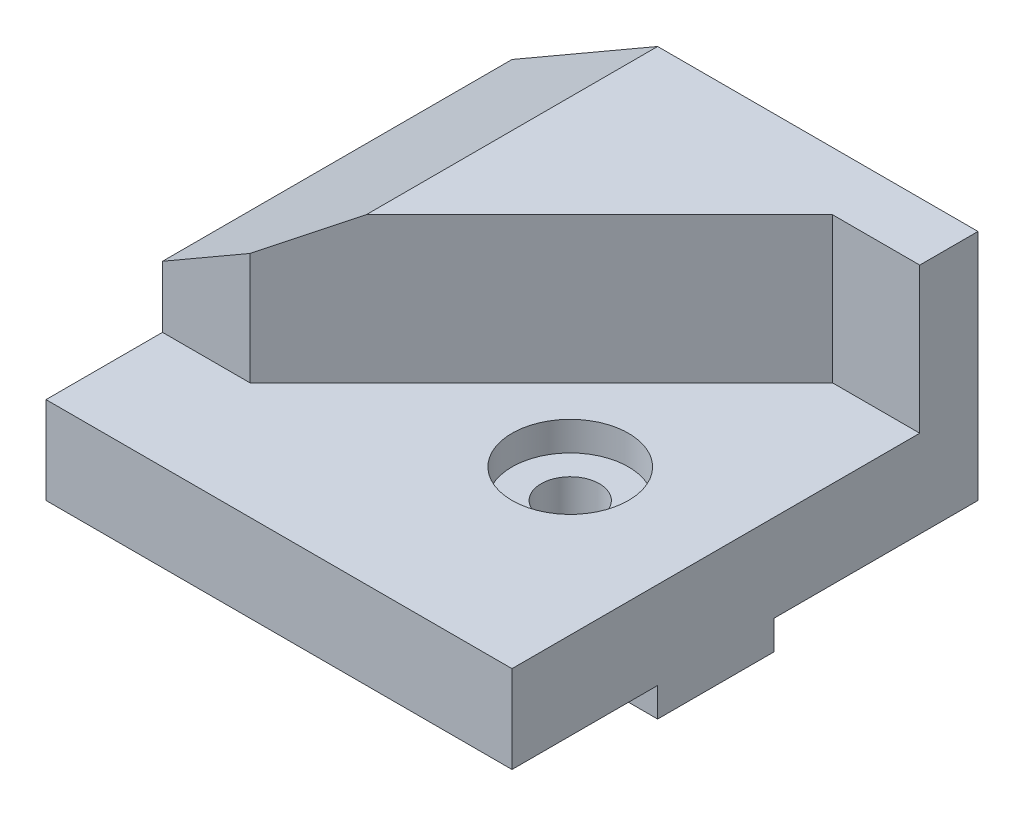
ISO-10303-21;
HEADER;
FILE_DESCRIPTION(('STEP AP214'),'2;1');
FILE_NAME('part.step','',(''),(''),'','','');
FILE_SCHEMA(('AUTOMOTIVE_DESIGN { 1 0 10303 214 1 1 1 1 }'));
ENDSEC;
DATA;
#1=APPLICATION_CONTEXT('core data for automotive mechanical design processes');
#2=APPLICATION_PROTOCOL_DEFINITION('international standard','automotive_design',2000,#1);
#3=PRODUCT_CONTEXT('',#1,'mechanical');
#4=PRODUCT('Part','Part','',(#3));
#5=PRODUCT_RELATED_PRODUCT_CATEGORY('part','',(#4));
#6=PRODUCT_DEFINITION_FORMATION('','',#4);
#7=PRODUCT_DEFINITION_CONTEXT('part definition',#1,'design');
#8=PRODUCT_DEFINITION('design','',#6,#7);
#9=PRODUCT_DEFINITION_SHAPE('','',#8);
#10=(LENGTH_UNIT() NAMED_UNIT(*) SI_UNIT(.MILLI.,.METRE.));
#11=(NAMED_UNIT(*) PLANE_ANGLE_UNIT() SI_UNIT($,.RADIAN.));
#12=(NAMED_UNIT(*) SI_UNIT($,.STERADIAN.) SOLID_ANGLE_UNIT());
#13=UNCERTAINTY_MEASURE_WITH_UNIT(LENGTH_MEASURE(1.E-05),#10,'distance_accuracy_value','');
#14=(GEOMETRIC_REPRESENTATION_CONTEXT(3) GLOBAL_UNCERTAINTY_ASSIGNED_CONTEXT((#13)) GLOBAL_UNIT_ASSIGNED_CONTEXT((#10,
#11,#12)) REPRESENTATION_CONTEXT('',''));
#15=CARTESIAN_POINT('',(0.,0.,0.));
#16=DIRECTION('',(0.,0.,1.));
#17=DIRECTION('',(1.,0.,0.));
#18=AXIS2_PLACEMENT_3D('',#15,#16,#17);
#19=CARTESIAN_POINT('',(15.,-45.,5.));
#20=DIRECTION('',(0.,1.,0.));
#21=DIRECTION('',(0.,0.,1.));
#22=AXIS2_PLACEMENT_3D('',#19,#20,#21);
#23=CYLINDRICAL_SURFACE('',#22,5.);
#24=CARTESIAN_POINT('',(15.,-5.,5.));
#25=DIRECTION('',(0.,-1.,0.));
#26=DIRECTION('',(0.,0.,-1.));
#27=AXIS2_PLACEMENT_3D('',#24,#25,#26);
#28=CIRCLE('',#27,5.);
#29=CARTESIAN_POINT('',(15.,-5.,0.));
#30=VERTEX_POINT('',#29);
#31=EDGE_CURVE('E202',#30,#30,#28,.T.);
#32=ORIENTED_EDGE('',*,*,#31,.T.);
#33=EDGE_LOOP('',(#32));
#34=FACE_BOUND('',#33,.T.);
#35=CARTESIAN_POINT('',(15.,9.99999999999999,5.));
#36=DIRECTION('',(0.,1.,0.));
#37=DIRECTION('',(0.,0.,1.));
#38=AXIS2_PLACEMENT_3D('',#35,#36,#37);
#39=CIRCLE('',#38,5.);
#40=CARTESIAN_POINT('',(15.,9.99999999999999,10.));
#41=VERTEX_POINT('',#40);
#42=EDGE_CURVE('E187',#41,#41,#39,.F.);
#43=ORIENTED_EDGE('',*,*,#42,.F.);
#44=EDGE_LOOP('',(#43));
#45=FACE_BOUND('',#44,.T.);
#46=ADVANCED_FACE('F44',(#34,#45),#23,.F.);
#47=CARTESIAN_POINT('',(0.,0.,0.));
#48=DIRECTION('',(0.,1.,0.));
#49=DIRECTION('',(0.,0.,1.));
#50=AXIS2_PLACEMENT_3D('',#47,#48,#49);
#51=PLANE('',#50);
#52=DIRECTION('',(-1.,0.,0.));
#53=VECTOR('',#52,1.);
#54=CARTESIAN_POINT('',(-40.,0.,15.));
#55=LINE('',#54,#53);
#56=CARTESIAN_POINT('',(40.,0.,15.));
#57=VERTEX_POINT('',#56);
#58=CARTESIAN_POINT('',(-40.,0.,15.));
#59=VERTEX_POINT('',#58);
#60=EDGE_CURVE('E194',#57,#59,#55,.T.);
#61=ORIENTED_EDGE('',*,*,#60,.F.);
#62=DIRECTION('',(0.,0.,-1.));
#63=VECTOR('',#62,1.);
#64=CARTESIAN_POINT('',(40.,0.,-40.));
#65=LINE('',#64,#63);
#66=CARTESIAN_POINT('',(40.,0.,40.));
#67=VERTEX_POINT('',#66);
#68=EDGE_CURVE('E227',#67,#57,#65,.T.);
#69=ORIENTED_EDGE('',*,*,#68,.F.);
#70=DIRECTION('',(1.,0.,0.));
#71=VECTOR('',#70,1.);
#72=CARTESIAN_POINT('',(-40.,0.,40.));
#73=LINE('',#72,#71);
#74=CARTESIAN_POINT('',(-40.,0.,40.));
#75=VERTEX_POINT('',#74);
#76=EDGE_CURVE('E224',#75,#67,#73,.T.);
#77=ORIENTED_EDGE('',*,*,#76,.F.);
#78=DIRECTION('',(0.,0.,1.));
#79=VECTOR('',#78,1.);
#80=CARTESIAN_POINT('',(-40.,0.,-40.));
#81=LINE('',#80,#79);
#82=EDGE_CURVE('E231',#59,#75,#81,.T.);
#83=ORIENTED_EDGE('',*,*,#82,.F.);
#84=EDGE_LOOP('',(#61,#69,#77,#83));
#85=FACE_BOUND('',#84,.T.);
#86=ADVANCED_FACE('F252',(#85),#51,.F.);
#87=DIRECTION('',(1.,0.,0.));
#88=VECTOR('',#87,1.);
#89=CARTESIAN_POINT('',(-40.,0.,-4.99999999999999));
#90=LINE('',#89,#88);
#91=CARTESIAN_POINT('',(-40.,0.,-4.99999999999999));
#92=VERTEX_POINT('',#91);
#93=CARTESIAN_POINT('',(40.,0.,-4.99999999999999));
#94=VERTEX_POINT('',#93);
#95=EDGE_CURVE('E205',#92,#94,#90,.T.);
#96=ORIENTED_EDGE('',*,*,#95,.F.);
#97=CARTESIAN_POINT('',(-40.,0.,-40.));
#98=VERTEX_POINT('',#97);
#99=EDGE_CURVE('E232',#98,#92,#81,.T.);
#100=ORIENTED_EDGE('',*,*,#99,.F.);
#101=DIRECTION('',(-1.,0.,0.));
#102=VECTOR('',#101,1.);
#103=CARTESIAN_POINT('',(-40.,0.,-40.));
#104=LINE('',#103,#102);
#105=CARTESIAN_POINT('',(40.,0.,-40.));
#106=VERTEX_POINT('',#105);
#107=EDGE_CURVE('E233',#106,#98,#104,.T.);
#108=ORIENTED_EDGE('',*,*,#107,.F.);
#109=EDGE_CURVE('E218',#94,#106,#65,.T.);
#110=ORIENTED_EDGE('',*,*,#109,.F.);
#111=EDGE_LOOP('',(#96,#100,#108,#110));
#112=FACE_BOUND('',#111,.T.);
#113=ADVANCED_FACE('F259',(#112),#51,.F.);
#114=CARTESIAN_POINT('',(40.,15.,-40.));
#115=DIRECTION('',(-1.,0.,0.));
#116=DIRECTION('',(0.,0.,1.));
#117=AXIS2_PLACEMENT_3D('',#114,#115,#116);
#118=PLANE('',#117);
#119=ORIENTED_EDGE('',*,*,#68,.T.);
#120=DIRECTION('',(0.,1.,0.));
#121=VECTOR('',#120,1.);
#122=CARTESIAN_POINT('',(40.,-5.,15.));
#123=LINE('',#122,#121);
#124=CARTESIAN_POINT('',(40.,-5.,15.));
#125=VERTEX_POINT('',#124);
#126=EDGE_CURVE('E209',#125,#57,#123,.T.);
#127=ORIENTED_EDGE('',*,*,#126,.F.);
#128=DIRECTION('',(0.,0.,1.));
#129=VECTOR('',#128,1.);
#130=CARTESIAN_POINT('',(40.,-5.,15.));
#131=LINE('',#130,#129);
#132=CARTESIAN_POINT('',(40.,-5.,-4.99999999999999));
#133=VERTEX_POINT('',#132);
#134=EDGE_CURVE('E197',#133,#125,#131,.T.);
#135=ORIENTED_EDGE('',*,*,#134,.F.);
#136=DIRECTION('',(0.,1.,0.));
#137=VECTOR('',#136,1.);
#138=CARTESIAN_POINT('',(40.,-5.,-4.99999999999999));
#139=LINE('',#138,#137);
#140=EDGE_CURVE('E213',#133,#94,#139,.T.);
#141=ORIENTED_EDGE('',*,*,#140,.T.);
#142=ORIENTED_EDGE('',*,*,#109,.T.);
#143=DIRECTION('',(0.,-1.,0.));
#144=VECTOR('',#143,1.);
#145=CARTESIAN_POINT('',(40.,15.,-40.));
#146=LINE('',#145,#144);
#147=CARTESIAN_POINT('',(40.,40.,-40.));
#148=VERTEX_POINT('',#147);
#149=EDGE_CURVE('E52',#148,#106,#146,.T.);
#150=ORIENTED_EDGE('',*,*,#149,.F.);
#151=DIRECTION('',(0.,0.,-1.));
#152=VECTOR('',#151,1.);
#153=CARTESIAN_POINT('',(40.,40.,-40.));
#154=LINE('',#153,#152);
#155=CARTESIAN_POINT('',(40.,40.,-30.));
#156=VERTEX_POINT('',#155);
#157=EDGE_CURVE('E160',#156,#148,#154,.T.);
#158=ORIENTED_EDGE('',*,*,#157,.F.);
#159=DIRECTION('',(0.,-1.,0.));
#160=VECTOR('',#159,1.);
#161=CARTESIAN_POINT('',(40.,40.,-30.));
#162=LINE('',#161,#160);
#163=CARTESIAN_POINT('',(40.,15.,-30.));
#164=VERTEX_POINT('',#163);
#165=EDGE_CURVE('E168',#156,#164,#162,.T.);
#166=ORIENTED_EDGE('',*,*,#165,.T.);
#167=DIRECTION('',(0.,0.,-1.));
#168=VECTOR('',#167,1.);
#169=CARTESIAN_POINT('',(40.,15.,-40.));
#170=LINE('',#169,#168);
#171=CARTESIAN_POINT('',(40.,15.,40.));
#172=VERTEX_POINT('',#171);
#173=EDGE_CURVE('E219',#172,#164,#170,.T.);
#174=ORIENTED_EDGE('',*,*,#173,.F.);
#175=DIRECTION('',(0.,-1.,0.));
#176=VECTOR('',#175,1.);
#177=CARTESIAN_POINT('',(40.,15.,40.));
#178=LINE('',#177,#176);
#179=EDGE_CURVE('E230',#172,#67,#178,.T.);
#180=ORIENTED_EDGE('',*,*,#179,.T.);
#181=EDGE_LOOP('',(#119,#127,#135,#141,#142,#150,#158,#166,#174,#180));
#182=FACE_BOUND('',#181,.T.);
#183=ADVANCED_FACE('F50',(#182),#118,.F.);
#184=CARTESIAN_POINT('',(-40.,15.,-40.));
#185=DIRECTION('',(0.,0.,1.));
#186=DIRECTION('',(1.,0.,0.));
#187=AXIS2_PLACEMENT_3D('',#184,#185,#186);
#188=PLANE('',#187);
#189=DIRECTION('',(0.,-1.,0.));
#190=VECTOR('',#189,1.);
#191=CARTESIAN_POINT('',(-40.,15.,-40.));
#192=LINE('',#191,#190);
#193=CARTESIAN_POINT('',(-40.,25.5662432702596,-40.));
#194=VERTEX_POINT('',#193);
#195=EDGE_CURVE('E151',#194,#98,#192,.T.);
#196=ORIENTED_EDGE('',*,*,#195,.F.);
#197=DIRECTION('',(-0.866025403784442,-0.499999999999995,0.));
#198=VECTOR('',#197,1.);
#199=CARTESIAN_POINT('',(-40.,25.5662432702596,-40.));
#200=LINE('',#199,#198);
#201=CARTESIAN_POINT('',(-15.,40.,-40.));
#202=VERTEX_POINT('',#201);
#203=EDGE_CURVE('E137',#202,#194,#200,.T.);
#204=ORIENTED_EDGE('',*,*,#203,.F.);
#205=DIRECTION('',(-1.,0.,0.));
#206=VECTOR('',#205,1.);
#207=CARTESIAN_POINT('',(40.,40.,-40.));
#208=LINE('',#207,#206);
#209=EDGE_CURVE('E149',#148,#202,#208,.T.);
#210=ORIENTED_EDGE('',*,*,#209,.F.);
#211=ORIENTED_EDGE('',*,*,#149,.T.);
#212=ORIENTED_EDGE('',*,*,#107,.T.);
#213=EDGE_LOOP('',(#196,#204,#210,#211,#212));
#214=FACE_BOUND('',#213,.T.);
#215=ADVANCED_FACE('F150',(#214),#188,.F.);
#216=CARTESIAN_POINT('',(-40.,15.,-40.));
#217=DIRECTION('',(1.,0.,0.));
#218=DIRECTION('',(0.,0.,-1.));
#219=AXIS2_PLACEMENT_3D('',#216,#217,#218);
#220=PLANE('',#219);
#221=DIRECTION('',(0.,-1.,0.));
#222=VECTOR('',#221,1.);
#223=CARTESIAN_POINT('',(-40.,40.,20.));
#224=LINE('',#223,#222);
#225=CARTESIAN_POINT('',(-40.,25.5662432702596,20.));
#226=VERTEX_POINT('',#225);
#227=CARTESIAN_POINT('',(-40.,15.,20.));
#228=VERTEX_POINT('',#227);
#229=EDGE_CURVE('E185',#226,#228,#224,.T.);
#230=ORIENTED_EDGE('',*,*,#229,.F.);
#231=DIRECTION('',(0.,0.,-1.));
#232=VECTOR('',#231,1.);
#233=CARTESIAN_POINT('',(-40.,25.5662432702596,60.));
#234=LINE('',#233,#232);
#235=EDGE_CURVE('E155',#226,#194,#234,.T.);
#236=ORIENTED_EDGE('',*,*,#235,.T.);
#237=ORIENTED_EDGE('',*,*,#195,.T.);
#238=ORIENTED_EDGE('',*,*,#99,.T.);
#239=DIRECTION('',(0.,1.,0.));
#240=VECTOR('',#239,1.);
#241=CARTESIAN_POINT('',(-40.,-5.,-4.99999999999999));
#242=LINE('',#241,#240);
#243=CARTESIAN_POINT('',(-40.,-5.,-4.99999999999999));
#244=VERTEX_POINT('',#243);
#245=EDGE_CURVE('E216',#244,#92,#242,.T.);
#246=ORIENTED_EDGE('',*,*,#245,.F.);
#247=DIRECTION('',(0.,0.,-1.));
#248=VECTOR('',#247,1.);
#249=CARTESIAN_POINT('',(-40.,-5.,15.));
#250=LINE('',#249,#248);
#251=CARTESIAN_POINT('',(-40.,-5.,15.));
#252=VERTEX_POINT('',#251);
#253=EDGE_CURVE('E193',#252,#244,#250,.T.);
#254=ORIENTED_EDGE('',*,*,#253,.F.);
#255=DIRECTION('',(0.,1.,0.));
#256=VECTOR('',#255,1.);
#257=CARTESIAN_POINT('',(-40.,-5.,15.));
#258=LINE('',#257,#256);
#259=EDGE_CURVE('E203',#252,#59,#258,.T.);
#260=ORIENTED_EDGE('',*,*,#259,.T.);
#261=ORIENTED_EDGE('',*,*,#82,.T.);
#262=DIRECTION('',(0.,-1.,0.));
#263=VECTOR('',#262,1.);
#264=CARTESIAN_POINT('',(-40.,15.,40.));
#265=LINE('',#264,#263);
#266=CARTESIAN_POINT('',(-40.,15.,40.));
#267=VERTEX_POINT('',#266);
#268=EDGE_CURVE('E238',#267,#75,#265,.T.);
#269=ORIENTED_EDGE('',*,*,#268,.F.);
#270=DIRECTION('',(0.,0.,1.));
#271=VECTOR('',#270,1.);
#272=CARTESIAN_POINT('',(-40.,15.,-40.));
#273=LINE('',#272,#271);
#274=EDGE_CURVE('E225',#228,#267,#273,.T.);
#275=ORIENTED_EDGE('',*,*,#274,.F.);
#276=EDGE_LOOP('',(#230,#236,#237,#238,#246,#254,#260,#261,#269,#275));
#277=FACE_BOUND('',#276,.T.);
#278=ADVANCED_FACE('F283',(#277),#220,.F.);
#279=CARTESIAN_POINT('',(-40.,15.,40.));
#280=DIRECTION('',(0.,0.,-1.));
#281=DIRECTION('',(-1.,0.,0.));
#282=AXIS2_PLACEMENT_3D('',#279,#280,#281);
#283=PLANE('',#282);
#284=ORIENTED_EDGE('',*,*,#76,.T.);
#285=ORIENTED_EDGE('',*,*,#179,.F.);
#286=DIRECTION('',(1.,0.,0.));
#287=VECTOR('',#286,1.);
#288=CARTESIAN_POINT('',(-40.,15.,40.));
#289=LINE('',#288,#287);
#290=EDGE_CURVE('E223',#267,#172,#289,.T.);
#291=ORIENTED_EDGE('',*,*,#290,.F.);
#292=ORIENTED_EDGE('',*,*,#268,.T.);
#293=EDGE_LOOP('',(#284,#285,#291,#292));
#294=FACE_BOUND('',#293,.T.);
#295=ADVANCED_FACE('F278',(#294),#283,.F.);
#296=CARTESIAN_POINT('',(0.,15.,0.));
#297=DIRECTION('',(0.,1.,0.));
#298=DIRECTION('',(0.,0.,1.));
#299=AXIS2_PLACEMENT_3D('',#296,#297,#298);
#300=PLANE('',#299);
#301=DIRECTION('',(1.,0.,0.));
#302=VECTOR('',#301,1.);
#303=CARTESIAN_POINT('',(40.,15.,-30.));
#304=LINE('',#303,#302);
#305=CARTESIAN_POINT('',(25.,15.,-30.));
#306=VERTEX_POINT('',#305);
#307=EDGE_CURVE('E70',#306,#164,#304,.T.);
#308=ORIENTED_EDGE('',*,*,#307,.F.);
#309=DIRECTION('',(0.707106781186547,0.,-0.707106781186547));
#310=VECTOR('',#309,1.);
#311=CARTESIAN_POINT('',(-25.,15.,20.));
#312=LINE('',#311,#310);
#313=CARTESIAN_POINT('',(-25.,15.,20.));
#314=VERTEX_POINT('',#313);
#315=EDGE_CURVE('E165',#314,#306,#312,.T.);
#316=ORIENTED_EDGE('',*,*,#315,.F.);
#317=DIRECTION('',(1.,0.,0.));
#318=VECTOR('',#317,1.);
#319=CARTESIAN_POINT('',(-40.,15.,20.));
#320=LINE('',#319,#318);
#321=EDGE_CURVE('E171',#228,#314,#320,.T.);
#322=ORIENTED_EDGE('',*,*,#321,.F.);
#323=ORIENTED_EDGE('',*,*,#274,.T.);
#324=ORIENTED_EDGE('',*,*,#290,.T.);
#325=ORIENTED_EDGE('',*,*,#173,.T.);
#326=EDGE_LOOP('',(#308,#316,#322,#323,#324,#325));
#327=FACE_BOUND('',#326,.T.);
#328=CARTESIAN_POINT('',(15.,15.,5.));
#329=DIRECTION('',(0.,1.,0.));
#330=DIRECTION('',(0.,0.,1.));
#331=AXIS2_PLACEMENT_3D('',#328,#329,#330);
#332=CIRCLE('',#331,10.);
#333=CARTESIAN_POINT('',(15.,15.,15.));
#334=VERTEX_POINT('',#333);
#335=EDGE_CURVE('E184',#334,#334,#332,.T.);
#336=ORIENTED_EDGE('',*,*,#335,.F.);
#337=EDGE_LOOP('',(#336));
#338=FACE_BOUND('',#337,.T.);
#339=ADVANCED_FACE('F280',(#327,#338),#300,.T.);
#340=CARTESIAN_POINT('',(-40.,-5.,-4.99999999999999));
#341=DIRECTION('',(0.,0.,1.));
#342=DIRECTION('',(1.,0.,0.));
#343=AXIS2_PLACEMENT_3D('',#340,#341,#342);
#344=PLANE('',#343);
#345=ORIENTED_EDGE('',*,*,#95,.T.);
#346=ORIENTED_EDGE('',*,*,#140,.F.);
#347=DIRECTION('',(1.,0.,0.));
#348=VECTOR('',#347,1.);
#349=CARTESIAN_POINT('',(-40.,-5.,-4.99999999999999));
#350=LINE('',#349,#348);
#351=EDGE_CURVE('E192',#244,#133,#350,.T.);
#352=ORIENTED_EDGE('',*,*,#351,.F.);
#353=ORIENTED_EDGE('',*,*,#245,.T.);
#354=EDGE_LOOP('',(#345,#346,#352,#353));
#355=FACE_BOUND('',#354,.T.);
#356=ADVANCED_FACE('F272',(#355),#344,.F.);
#357=CARTESIAN_POINT('',(-40.,-5.,15.));
#358=DIRECTION('',(0.,0.,-1.));
#359=DIRECTION('',(-1.,0.,0.));
#360=AXIS2_PLACEMENT_3D('',#357,#358,#359);
#361=PLANE('',#360);
#362=ORIENTED_EDGE('',*,*,#60,.T.);
#363=ORIENTED_EDGE('',*,*,#259,.F.);
#364=DIRECTION('',(-1.,0.,0.));
#365=VECTOR('',#364,1.);
#366=CARTESIAN_POINT('',(-40.,-5.,15.));
#367=LINE('',#366,#365);
#368=EDGE_CURVE('E200',#125,#252,#367,.T.);
#369=ORIENTED_EDGE('',*,*,#368,.F.);
#370=ORIENTED_EDGE('',*,*,#126,.T.);
#371=EDGE_LOOP('',(#362,#363,#369,#370));
#372=FACE_BOUND('',#371,.T.);
#373=ADVANCED_FACE('F267',(#372),#361,.F.);
#374=CARTESIAN_POINT('',(0.,-5.,0.));
#375=DIRECTION('',(0.,-1.,0.));
#376=DIRECTION('',(0.,0.,-1.));
#377=AXIS2_PLACEMENT_3D('',#374,#375,#376);
#378=PLANE('',#377);
#379=ORIENTED_EDGE('',*,*,#31,.F.);
#380=EDGE_LOOP('',(#379));
#381=FACE_BOUND('',#380,.T.);
#382=ORIENTED_EDGE('',*,*,#253,.T.);
#383=ORIENTED_EDGE('',*,*,#351,.T.);
#384=ORIENTED_EDGE('',*,*,#134,.T.);
#385=ORIENTED_EDGE('',*,*,#368,.T.);
#386=EDGE_LOOP('',(#382,#383,#384,#385));
#387=FACE_BOUND('',#386,.T.);
#388=ADVANCED_FACE('F266',(#381,#387),#378,.T.);
#389=CARTESIAN_POINT('',(15.,10.,5.));
#390=DIRECTION('',(0.,1.,0.));
#391=DIRECTION('',(0.,0.,1.));
#392=AXIS2_PLACEMENT_3D('',#389,#390,#391);
#393=PLANE('',#392);
#394=CARTESIAN_POINT('',(15.,10.,5.));
#395=DIRECTION('',(0.,1.,0.));
#396=DIRECTION('',(0.,0.,1.));
#397=AXIS2_PLACEMENT_3D('',#394,#395,#396);
#398=CIRCLE('',#397,10.);
#399=CARTESIAN_POINT('',(15.,10.,15.));
#400=VERTEX_POINT('',#399);
#401=EDGE_CURVE('E183',#400,#400,#398,.T.);
#402=ORIENTED_EDGE('',*,*,#401,.T.);
#403=EDGE_LOOP('',(#402));
#404=FACE_BOUND('',#403,.T.);
#405=ORIENTED_EDGE('',*,*,#42,.T.);
#406=EDGE_LOOP('',(#405));
#407=FACE_BOUND('',#406,.T.);
#408=ADVANCED_FACE('F247',(#404,#407),#393,.T.);
#409=CARTESIAN_POINT('',(15.,10.,5.));
#410=DIRECTION('',(0.,1.,0.));
#411=DIRECTION('',(0.,0.,1.));
#412=AXIS2_PLACEMENT_3D('',#409,#410,#411);
#413=CYLINDRICAL_SURFACE('',#412,10.);
#414=ORIENTED_EDGE('',*,*,#401,.F.);
#415=EDGE_LOOP('',(#414));
#416=FACE_BOUND('',#415,.T.);
#417=ORIENTED_EDGE('',*,*,#335,.T.);
#418=EDGE_LOOP('',(#417));
#419=FACE_BOUND('',#418,.T.);
#420=ADVANCED_FACE('F262',(#416,#419),#413,.F.);
#421=CARTESIAN_POINT('',(-40.,40.,20.));
#422=DIRECTION('',(0.,0.,-1.));
#423=DIRECTION('',(-1.,0.,0.));
#424=AXIS2_PLACEMENT_3D('',#421,#422,#423);
#425=PLANE('',#424);
#426=DIRECTION('',(0.,-1.,0.));
#427=VECTOR('',#426,1.);
#428=CARTESIAN_POINT('',(-25.,40.,20.));
#429=LINE('',#428,#427);
#430=CARTESIAN_POINT('',(-25.,34.2264973081038,20.));
#431=VERTEX_POINT('',#430);
#432=EDGE_CURVE('E179',#431,#314,#429,.T.);
#433=ORIENTED_EDGE('',*,*,#432,.F.);
#434=DIRECTION('',(-0.866025403784442,-0.499999999999995,0.));
#435=VECTOR('',#434,1.);
#436=CARTESIAN_POINT('',(-33.7500000000001,29.1746824526946,20.));
#437=LINE('',#436,#435);
#438=EDGE_CURVE('E164',#431,#226,#437,.T.);
#439=ORIENTED_EDGE('',*,*,#438,.T.);
#440=ORIENTED_EDGE('',*,*,#229,.T.);
#441=ORIENTED_EDGE('',*,*,#321,.T.);
#442=EDGE_LOOP('',(#433,#439,#440,#441));
#443=FACE_BOUND('',#442,.T.);
#444=ADVANCED_FACE('F326',(#443),#425,.F.);
#445=CARTESIAN_POINT('',(-25.,40.,20.));
#446=DIRECTION('',(-0.707106781186547,0.,-0.707106781186547));
#447=DIRECTION('',(-0.707106781186548,0.,0.707106781186548));
#448=AXIS2_PLACEMENT_3D('',#445,#446,#447);
#449=PLANE('',#448);
#450=DIRECTION('',(0.707106781186547,0.,-0.707106781186547));
#451=VECTOR('',#450,1.);
#452=CARTESIAN_POINT('',(-25.,40.,20.));
#453=LINE('',#452,#451);
#454=CARTESIAN_POINT('',(-15.,40.,10.));
#455=VERTEX_POINT('',#454);
#456=CARTESIAN_POINT('',(25.,40.,-30.));
#457=VERTEX_POINT('',#456);
#458=EDGE_CURVE('E158',#455,#457,#453,.T.);
#459=ORIENTED_EDGE('',*,*,#458,.F.);
#460=DIRECTION('',(-0.654653670707979,-0.377964473009223,0.654653670707979));
#461=VECTOR('',#460,1.);
#462=CARTESIAN_POINT('',(-23.5714285714286,35.0512834069461,18.5714285714286));
#463=LINE('',#462,#461);
#464=EDGE_CURVE('E56',#455,#431,#463,.T.);
#465=ORIENTED_EDGE('',*,*,#464,.T.);
#466=ORIENTED_EDGE('',*,*,#432,.T.);
#467=ORIENTED_EDGE('',*,*,#315,.T.);
#468=DIRECTION('',(0.,-1.,0.));
#469=VECTOR('',#468,1.);
#470=CARTESIAN_POINT('',(25.,40.,-30.));
#471=LINE('',#470,#469);
#472=EDGE_CURVE('E180',#457,#306,#471,.T.);
#473=ORIENTED_EDGE('',*,*,#472,.F.);
#474=EDGE_LOOP('',(#459,#465,#466,#467,#473));
#475=FACE_BOUND('',#474,.T.);
#476=ADVANCED_FACE('F319',(#475),#449,.F.);
#477=CARTESIAN_POINT('',(40.,40.,-30.));
#478=DIRECTION('',(0.,0.,-1.));
#479=DIRECTION('',(-1.,0.,0.));
#480=AXIS2_PLACEMENT_3D('',#477,#478,#479);
#481=PLANE('',#480);
#482=ORIENTED_EDGE('',*,*,#307,.T.);
#483=ORIENTED_EDGE('',*,*,#165,.F.);
#484=DIRECTION('',(1.,0.,0.));
#485=VECTOR('',#484,1.);
#486=CARTESIAN_POINT('',(40.,40.,-30.));
#487=LINE('',#486,#485);
#488=EDGE_CURVE('E159',#457,#156,#487,.T.);
#489=ORIENTED_EDGE('',*,*,#488,.F.);
#490=ORIENTED_EDGE('',*,*,#472,.T.);
#491=EDGE_LOOP('',(#482,#483,#489,#490));
#492=FACE_BOUND('',#491,.T.);
#493=ADVANCED_FACE('F320',(#492),#481,.F.);
#494=CARTESIAN_POINT('',(0.,40.,0.));
#495=DIRECTION('',(0.,1.,0.));
#496=DIRECTION('',(0.,0.,1.));
#497=AXIS2_PLACEMENT_3D('',#494,#495,#496);
#498=PLANE('',#497);
#499=DIRECTION('',(0.,0.,-1.));
#500=VECTOR('',#499,1.);
#501=CARTESIAN_POINT('',(-15.,40.,0.));
#502=LINE('',#501,#500);
#503=EDGE_CURVE('E11',#455,#202,#502,.T.);
#504=ORIENTED_EDGE('',*,*,#503,.F.);
#505=ORIENTED_EDGE('',*,*,#458,.T.);
#506=ORIENTED_EDGE('',*,*,#488,.T.);
#507=ORIENTED_EDGE('',*,*,#157,.T.);
#508=ORIENTED_EDGE('',*,*,#209,.T.);
#509=EDGE_LOOP('',(#504,#505,#506,#507,#508));
#510=FACE_BOUND('',#509,.T.);
#511=ADVANCED_FACE('F154',(#510),#498,.T.);
#512=CARTESIAN_POINT('',(-40.,25.5662432702596,60.));
#513=DIRECTION('',(0.499999999999995,-0.866025403784442,0.));
#514=DIRECTION('',(0.866025403784442,0.499999999999995,0.));
#515=AXIS2_PLACEMENT_3D('',#512,#513,#514);
#516=PLANE('',#515);
#517=ORIENTED_EDGE('',*,*,#464,.F.);
#518=ORIENTED_EDGE('',*,*,#503,.T.);
#519=ORIENTED_EDGE('',*,*,#203,.T.);
#520=ORIENTED_EDGE('',*,*,#235,.F.);
#521=ORIENTED_EDGE('',*,*,#438,.F.);
#522=EDGE_LOOP('',(#517,#518,#519,#520,#521));
#523=FACE_BOUND('',#522,.T.);
#524=ADVANCED_FACE('F136',(#523),#516,.F.);
#525=CLOSED_SHELL('',(#46,#86,#113,#183,#215,#278,#295,#339,#356,#373,#388,#408,#420,#444,#476,
#493,#511,#524));
#526=MANIFOLD_SOLID_BREP('B2',#525);
#527=ADVANCED_BREP_SHAPE_REPRESENTATION('',(#18,#526),#14);
#528=SHAPE_DEFINITION_REPRESENTATION(#9,#527);
ENDSEC;
END-ISO-10303-21;
